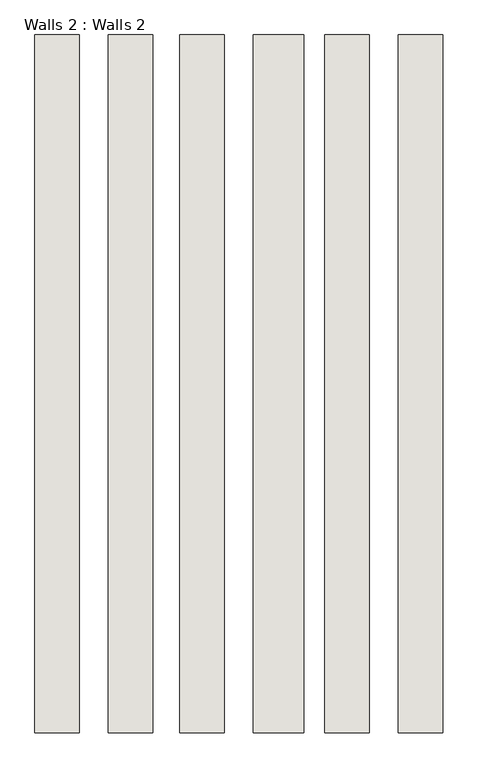
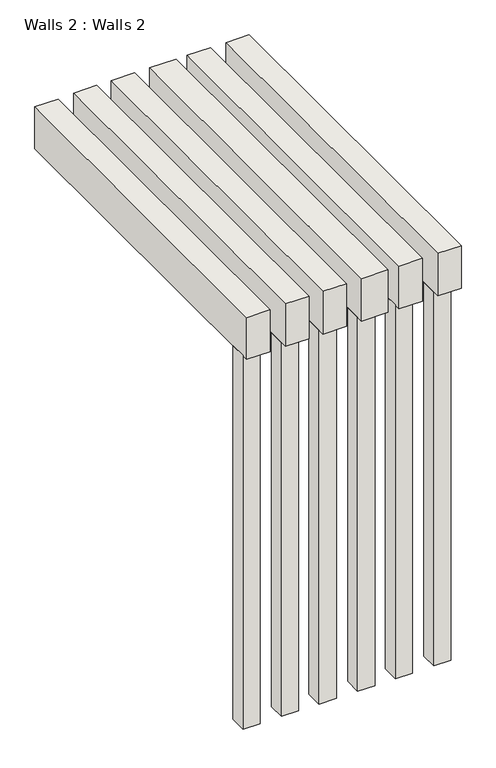
"""IFC4 building model written with IfcOpenShell, lengths in millimetres: wall geometry, Walls 2 : Walls 2."""

from ifc_helpers import new_model, si_unit, frame, origin, place, context, project, spatial, polyline, outline, extrude, source, transform, mapped, element, save


def walls_2_walls_2_a9f40376(model_context):
    return source(origin(), model_context, "Body", "SweptSolid", [
        extrude(outline(polyline([(-6243.9061529, -224.2825129), (-6345.5061529, -224.2825129), (-6345.5061529, -122.6825129), (-6243.9061529, -122.6825129), (-6243.9061529, -224.2825129)])), frame((0.0, 0.0, 6096.0), z_axis=(0.0, 0.0, 1.0), x_axis=(1.0, 0.0, 0.0)), (0.0, 0.0, 1.0), 2336.8),
        extrude(outline(polyline([(-6015.3061529, -224.2825129), (-6116.9061529, -224.2825129), (-6116.9061529, -122.6825129), (-6015.3061529, -122.6825129), (-6015.3061529, -224.2825129)])), frame((0.0, 0.0, 6096.0), z_axis=(0.0, 0.0, 1.0), x_axis=(1.0, 0.0, 0.0)), (0.0, 0.0, 1.0), 2336.8),
        extrude(outline(polyline([(-5793.0561529, -224.2825129), (-5894.6561529, -224.2825129), (-5894.6561529, -122.6825129), (-5793.0561529, -122.6825129), (-5793.0561529, -224.2825129)])), frame((0.0, 0.0, 6096.0), z_axis=(0.0, 0.0, 1.0), x_axis=(1.0, 0.0, 0.0)), (0.0, 0.0, 1.0), 2336.8),
        extrude(outline(polyline([(-5564.4561529, -224.2825129), (-5666.0561529, -224.2825129), (-5666.0561529, -122.6825129), (-5564.4561529, -122.6825129), (-5564.4561529, -224.2825129)])), frame((0.0, 0.0, 6096.0), z_axis=(0.0, 0.0, 1.0), x_axis=(1.0, 0.0, 0.0)), (0.0, 0.0, 1.0), 2336.8),
        extrude(outline(polyline([(-5342.2061529, -224.2825129), (-5443.8061529, -224.2825129), (-5443.8061529, -122.6825129), (-5342.2061529, -122.6825129), (-5342.2061529, -224.2825129)])), frame((0.0, 0.0, 6096.0), z_axis=(0.0, 0.0, 1.0), x_axis=(1.0, 0.0, 0.0)), (0.0, 0.0, 1.0), 2336.8),
        extrude(outline(polyline([(-5113.6061529, -224.2825129), (-5215.2061529, -224.2825129), (-5215.2061529, -122.6825129), (-5113.6061529, -122.6825129), (-5113.6061529, -224.2825129)])), frame((0.0, 0.0, 6096.0), z_axis=(0.0, 0.0, 1.0), x_axis=(1.0, 0.0, 0.0)), (0.0, 0.0, 1.0), 2336.8),
        extrude(outline(polyline([(-6207.1069291, -263.8046951), (-6345.5061529, -263.8046951), (-6345.5061529, 1907.6881753), (-6207.1069291, 1907.6881753), (-6207.1069291, -263.8046951)])), frame((0.0, 0.0, 8432.8), z_axis=(0.0, 0.0, 1.0), x_axis=(1.0, 0.0, 0.0)), (0.0, 0.0, 1.0), 260.35),
        extrude(outline(polyline([(-5978.5069291, -263.8046951), (-6116.9061529, -263.8046951), (-6116.9061529, 1907.6881753), (-5978.5069291, 1907.6881753), (-5978.5069291, -263.8046951)])), frame((0.0, 0.0, 8432.8), z_axis=(0.0, 0.0, 1.0), x_axis=(1.0, 0.0, 0.0)), (0.0, 0.0, 1.0), 266.7),
        extrude(outline(polyline([(-5756.2569291, -263.8046951), (-5894.6561529, -263.8046951), (-5894.6561529, 1907.6881753), (-5756.2569291, 1907.6881753), (-5756.2569291, -263.8046951)])), frame((0.0, 0.0, 8432.8), z_axis=(0.0, 0.0, 1.0), x_axis=(1.0, 0.0, 0.0)), (0.0, 0.0, 1.0), 266.7),
        extrude(outline(polyline([(-5508.6069291, -263.8046951), (-5666.0561529, -263.8046951), (-5666.0561529, 1907.6881753), (-5508.6069291, 1907.6881753), (-5508.6069291, -263.8046951)])), frame((0.0, 0.0, 8432.8), z_axis=(0.0, 0.0, 1.0), x_axis=(1.0, 0.0, 0.0)), (0.0, 0.0, 1.0), 266.7),
        extrude(outline(polyline([(-5305.4069291, -263.8046951), (-5443.8061529, -263.8046951), (-5443.8061529, 1907.6881753), (-5305.4069291, 1907.6881753), (-5305.4069291, -263.8046951)])), frame((0.0, 0.0, 8432.8), z_axis=(0.0, 0.0, 1.0), x_axis=(1.0, 0.0, 0.0)), (0.0, 0.0, 1.0), 266.7),
        extrude(outline(polyline([(-5076.8069291, -263.8046951), (-5215.2061529, -263.8046951), (-5215.2061529, 1907.6881753), (-5076.8069291, 1907.6881753), (-5076.8069291, -263.8046951)])), frame((0.0, 0.0, 8432.8), z_axis=(0.0, 0.0, 1.0), x_axis=(1.0, 0.0, 0.0)), (0.0, 0.0, 1.0), 266.7),
    ])


if __name__ == "__main__":
    model = new_model("IFC4")
    model_context = context("Model", 3, world=origin())
    ifc_project = project(units=[si_unit("LENGTHUNIT", "METRE", prefix="MILLI")], contexts=[model_context])
    site = spatial("IfcSite", under=ifc_project)
    building = spatial("IfcBuilding", under=site)
    placement = place(None, origin())
    walls_2_walls_2_shape = walls_2_walls_2_a9f40376(model_context)
    element("IfcWall", 1, ObjectType="Walls 2 : Walls 2", at=placement, inside=building, context=model_context, shape_type="MappedRepresentation", body=[
        mapped(walls_2_walls_2_shape, transform((0.0, 0.0, 0.0), x_axis=(1.0, 0.0, 0.0), y_axis=(0.0, 1.0, 0.0), z_axis=(0.0, 0.0, 1.0))),
    ])
    save(model, "model.ifc")

# Revit data of these elements
# Element 1 (IfcWall, "Walls 2 : Walls 2")
#   Materials on its faces: "1 white", "Default Wall"
# Materials
#   "1 white": class "Generic", colour RGB 244 245 241, transparency 0, Cost = 0
#   "Default Wall": colour RGB 128 128 128, transparency 0, Cost = 0
